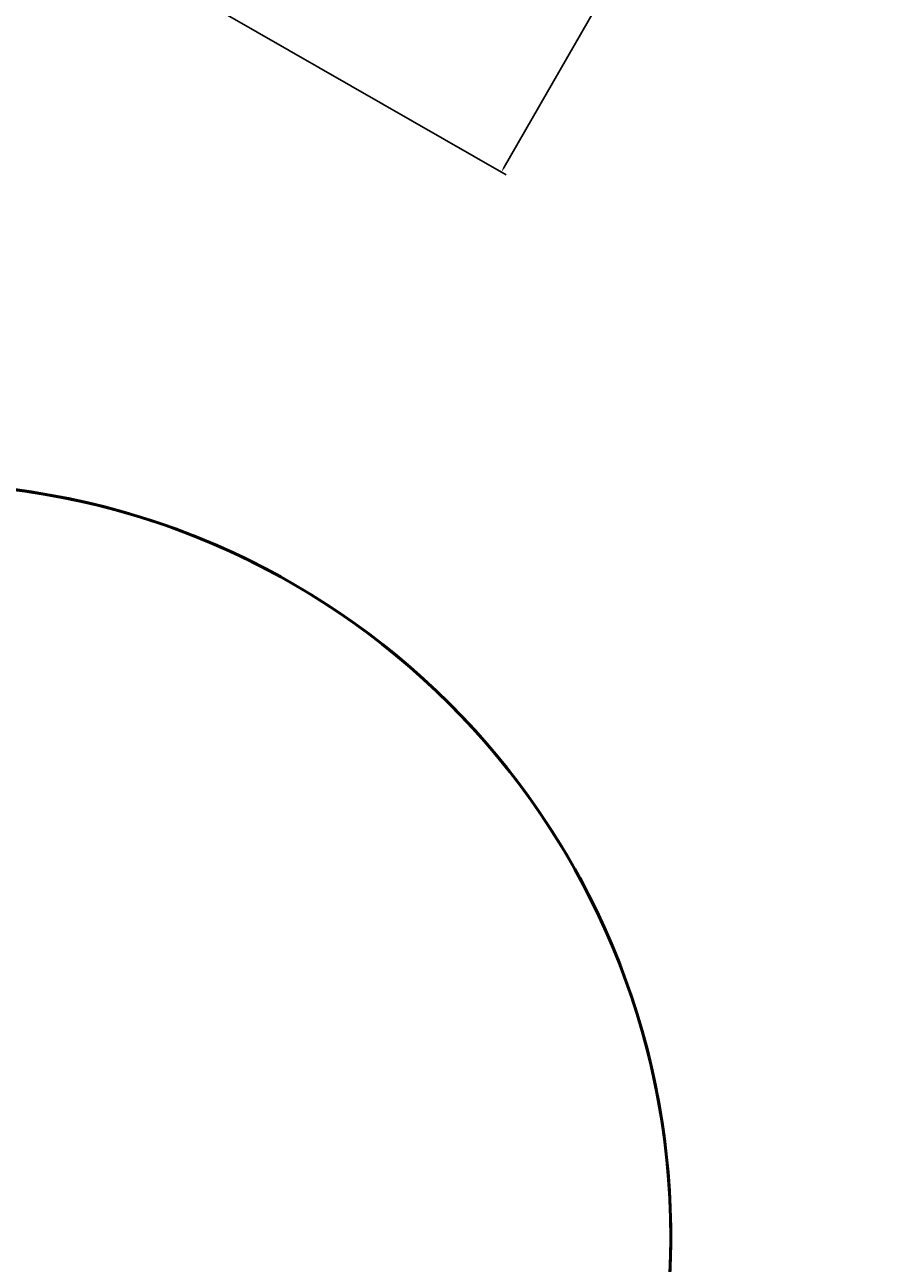
# Model space of a CAD drawing. Units: inches. Extents: x -99 to 284, y -92 to 134.
# Tile 6 of 16: x 36 to 64, y 14 to 55. Entities that reach past the tile are written whole.
import ezdxf

# ---------------------------------------------------------------- set-up
doc = ezdxf.new("R2010")
doc.units = ezdxf.units.IN
doc.header["$MEASUREMENT"] = 0
doc.layers.add('M-DIMS', color=2, linetype='Continuous', lineweight=18)
doc.layers.add('M-OUTL', color=7, linetype='Continuous', lineweight=50)
doc.styles.get("Standard").update_dxf_attribs({"font": 'arial.ttf'})
doc.dimstyles.get("Standard").update_dxf_attribs({"dimtxt": 0.18, "dimasz": 0.18, "dimexe": 0.18, "dimexo": 0.0625, "dimgap": 0.09, "dimtad": 0, "dimtih": 1, "dimtoh": 1, "dimdec": 4, "dimzin": 0, "dimdsep": 46, "dimtxsty": 'Standard', "dimcen": 0.09, "dimadec": 0, "dimazin": 0, "dimtfac": 1, "dimtdec": 4, "dimtofl": 0, "dimtmove": 0, "dimatfit": 3, "dimfxl": 1, "dimtolj": 1, "dimtzin": 0, "dimarcsym": 0})

# ---------------------------------------------------------------- blocks, each defined once
blk = doc.blocks.new('*D14')
at = {"layer": 'Defpoints', "color": 0, "transparency": 16777216}
for p in [(49.317, 79.47), (37.182, 58.303), (51.366, 50.171)]:
    blk.add_point(p, dxfattribs=at)
at = {"layer": 'M-DIMS', "color": 0, "lineweight": -2, "transparency": 16777216}
for p, q in [((49.371, 79.439), (63.657, 71.248)), ((63.412, 71.181), (57.537, 60.935)), ((51.455, 50.327), (57.33, 60.574)), ((37.236, 58.272), (51.522, 50.082))]:
    blk.add_line(p, q, dxfattribs=at)
at = {"layer": 'M-DIMS', "color": 0, "transparency": 16777216}
for points in [[(63.385, 71.196), (63.438, 71.167), (63.501, 71.338)], [(51.429, 50.342), (51.481, 50.312), (51.366, 50.171)]]:
    blk.add_solid(points, dxfattribs=at)
at = {"layer": 'M-DIMS', "color": 0, "transparency": 16777216, "insert": (57.433, 60.754), "char_height": 0.18, "attachment_point": 5}
blk.add_mtext('\\A1;24.4', dxfattribs=at)
blk = doc.blocks.new('*D19')
at = {"layer": 'Defpoints', "color": 0, "transparency": 16777216}
for p in [(112.982, 51.721), (-49.029, -22.013)]:
    blk.add_point(p, dxfattribs=at)
at = {"layer": 'M-DIMS', "color": 0, "lineweight": -2, "transparency": 16777216}
for p, q in [((31.886, 14.854), (32.066, 14.854)), ((31.976, 14.764), (31.976, 14.944)), ((-97.632, -44.133), (-49.192, -22.088)), ((-97.812, -44.133), (-97.632, -44.133))]:
    blk.add_line(p, q, dxfattribs=at)
at = {"layer": 'M-DIMS', "color": 0, "transparency": 16777216}
blk.add_solid([(-49.205, -22.06), (-49.18, -22.115), (-49.029, -22.013)], dxfattribs=at)
at = {"layer": 'M-DIMS', "color": 0, "transparency": 16777216, "insert": (-98.199, -44.133), "char_height": 0.18, "attachment_point": 5}
blk.add_mtext('\\A1;∅178', dxfattribs=at)
blk = doc.blocks.new('*D20')
at = {"layer": 'Defpoints', "color": 0, "transparency": 16777216}
for p in [(-35.23, 65.245), (99.183, -35.537)]:
    blk.add_point(p, dxfattribs=at)
at = {"layer": 'M-DIMS', "color": 0, "lineweight": -2, "transparency": 16777216}
for p, q in [((31.886, 14.854), (32.066, 14.854)), ((31.976, 14.764), (31.976, 14.944)), ((139.507, -65.772), (99.327, -35.645)), ((139.687, -65.772), (139.507, -65.772))]:
    blk.add_line(p, q, dxfattribs=at)
at = {"layer": 'M-DIMS', "color": 0, "transparency": 16777216}
blk.add_solid([(99.345, -35.621), (99.309, -35.669), (99.183, -35.537)], dxfattribs=at)
at = {"layer": 'M-DIMS', "color": 0, "transparency": 16777216, "insert": (140.074, -65.772), "char_height": 0.18, "attachment_point": 5}
blk.add_mtext('\\A1;∅168', dxfattribs=at)
blk = doc.blocks.new('*D21')
at = {"layer": 'Defpoints', "color": 0, "transparency": 16777216}
for p in [(19.926, 36.758), (44.027, -7.05)]:
    blk.add_point(p, dxfattribs=at)
at = {"layer": 'M-DIMS', "color": 0, "lineweight": -2, "transparency": 16777216}
for p, q in [((31.886, 14.854), (32.066, 14.854)), ((31.976, 14.764), (31.976, 14.944)), ((51.258, -20.192), (44.114, -7.208)), ((51.438, -20.192), (51.258, -20.192))]:
    blk.add_line(p, q, dxfattribs=at)
at = {"layer": 'M-DIMS', "color": 0, "transparency": 16777216}
blk.add_solid([(44.14, -7.193), (44.088, -7.222), (44.027, -7.05)], dxfattribs=at)
at = {"layer": 'M-DIMS', "color": 0, "transparency": 16777216, "insert": (51.755, -20.192), "char_height": 0.18, "attachment_point": 5}
blk.add_mtext('\\A1;∅50', dxfattribs=at)
blk = doc.blocks.new('*D22')
at = {"layer": 'Defpoints', "color": 0, "transparency": 16777216}
for p in [(39, 89.203), (31.976, 14.854)]:
    blk.add_point(p, dxfattribs=at)
at = {"layer": 'M-DIMS', "color": 0, "lineweight": -2, "transparency": 16777216}
for p, q in [((43.215, 133.813), (39.017, 89.383)), ((43.395, 133.813), (43.215, 133.813)), ((31.886, 14.854), (32.066, 14.854)), ((31.976, 14.764), (31.976, 14.944))]:
    blk.add_line(p, q, dxfattribs=at)
at = {"layer": 'M-DIMS', "color": 0, "transparency": 16777216}
blk.add_solid([(38.987, 89.385), (39.047, 89.38), (39, 89.203)], dxfattribs=at)
at = {"layer": 'M-DIMS', "color": 0, "transparency": 16777216, "insert": (44.068, 133.813), "char_height": 0.18, "attachment_point": 5}
blk.add_mtext('\\A1;5X R74.68', dxfattribs=at)

msp = doc.modelspace()

# ---------------------------------------------------------------- linework, layer by layer
at = {"layer": 'M-OUTL'}
for radius in [89, 84, 25]:
    msp.add_circle((31.9765, 14.8539), radius, dxfattribs=at)
msp.add_arc((31.9765, 14.8539), 25, 96.8921, 83.1079, dxfattribs=at)

# ---------------------------------------------------------------- dimensions: what is measured, and where the dimension line sits
at = {"layer": 'M-DIMS'}
dim = msp.add_radius_dim(center=(31.9765, 14.8539), mpoint=(39.0003, 89.2035), text='5X <>', dimstyle='Standard', override={"dimdec": 2, "dimlfac": 1, "dimrnd": 0, "dimzin": 0, "dimdsep": 46, "dimlunit": 2}, dxfattribs=at)
dim.commit()
dim.dimension.update_dxf_attribs({"geometry": '*D22', "text_midpoint": (44.068, 133.8132), "dimtype": 164})
dim = msp.add_linear_dim(base=(51.3659, 50.1711), p1=(49.3168, 79.4697), p2=(37.1817, 58.3032), angle=240.17365, dimstyle='Standard', override={"dimdec": 1, "dimlfac": 1, "dimrnd": 0, "dimzin": 0, "dimdsep": 46, "dimlunit": 2}, dxfattribs=at)
dim.commit()
dim.dimension.update_dxf_attribs({"geometry": '*D14', "text_midpoint": (57.4335, 60.7544)})
for p1, p2, picture, middle in [((-35.2301, 65.2451), (99.1831, -35.5373), '*D20', (140.074, -65.772)), ((112.9816, 51.7208), (-49.0286, -22.013), '*D19', (-98.1987, -44.1332)), ((19.9255, 36.7577), (44.0274, -7.0499), '*D21', (51.7545, -20.1921))]:
    dim = msp.add_diameter_dim_2p(p1=p1, p2=p2, dimstyle='Standard', override={"dimdec": 0, "dimlfac": 1, "dimrnd": 0, "dimzin": 0, "dimdsep": 46, "dimlunit": 2}, dxfattribs=at)
    dim.commit()
    dim.dimension.update_dxf_attribs({"geometry": picture, "text_midpoint": middle, "dimtype": 163})

doc.saveas('drawing.dxf')
